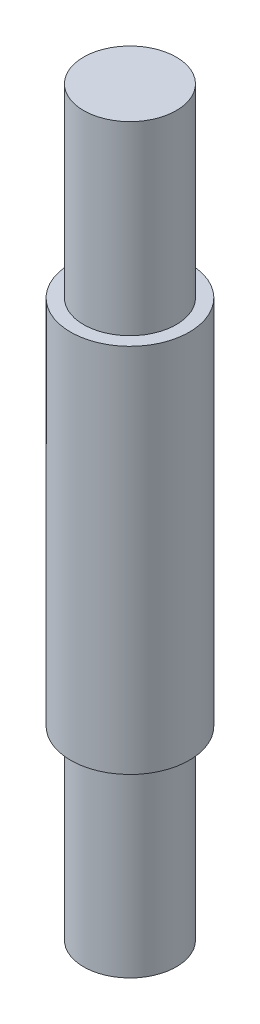
ISO-10303-21;
HEADER;
FILE_DESCRIPTION(('STEP AP214'),'2;1');
FILE_NAME('part.step','',(''),(''),'','','');
FILE_SCHEMA(('AUTOMOTIVE_DESIGN { 1 0 10303 214 1 1 1 1 }'));
ENDSEC;
DATA;
#1=APPLICATION_CONTEXT('core data for automotive mechanical design processes');
#2=APPLICATION_PROTOCOL_DEFINITION('international standard','automotive_design',2000,#1);
#3=PRODUCT_CONTEXT('',#1,'mechanical');
#4=PRODUCT('Part','Part','',(#3));
#5=PRODUCT_RELATED_PRODUCT_CATEGORY('part','',(#4));
#6=PRODUCT_DEFINITION_FORMATION('','',#4);
#7=PRODUCT_DEFINITION_CONTEXT('part definition',#1,'design');
#8=PRODUCT_DEFINITION('design','',#6,#7);
#9=PRODUCT_DEFINITION_SHAPE('','',#8);
#10=(LENGTH_UNIT() NAMED_UNIT(*) SI_UNIT(.MILLI.,.METRE.));
#11=(NAMED_UNIT(*) PLANE_ANGLE_UNIT() SI_UNIT($,.RADIAN.));
#12=(NAMED_UNIT(*) SI_UNIT($,.STERADIAN.) SOLID_ANGLE_UNIT());
#13=UNCERTAINTY_MEASURE_WITH_UNIT(LENGTH_MEASURE(1.E-05),#10,'distance_accuracy_value','');
#14=(GEOMETRIC_REPRESENTATION_CONTEXT(3) GLOBAL_UNCERTAINTY_ASSIGNED_CONTEXT((#13)) GLOBAL_UNIT_ASSIGNED_CONTEXT((#10,
#11,#12)) REPRESENTATION_CONTEXT('',''));
#15=CARTESIAN_POINT('',(0.,0.,0.));
#16=DIRECTION('',(0.,0.,1.));
#17=DIRECTION('',(1.,0.,0.));
#18=AXIS2_PLACEMENT_3D('',#15,#16,#17);
#19=CARTESIAN_POINT('',(0.,0.,0.));
#20=DIRECTION('',(0.,1.,0.));
#21=DIRECTION('',(-1.,0.,0.));
#22=AXIS2_PLACEMENT_3D('',#19,#20,#21);
#23=PLANE('',#22);
#24=CARTESIAN_POINT('',(0.,0.,0.));
#25=DIRECTION('',(0.,1.,0.));
#26=DIRECTION('',(-1.,0.,0.));
#27=AXIS2_PLACEMENT_3D('',#24,#25,#26);
#28=CIRCLE('',#27,12.5);
#29=CARTESIAN_POINT('',(-12.5,0.,0.));
#30=VERTEX_POINT('',#29);
#31=EDGE_CURVE('E10',#30,#30,#28,.T.);
#32=ORIENTED_EDGE('',*,*,#31,.F.);
#33=EDGE_LOOP('',(#32));
#34=FACE_BOUND('',#33,.T.);
#35=ADVANCED_FACE('F40',(#34),#23,.F.);
#36=CARTESIAN_POINT('',(0.,200.,0.));
#37=DIRECTION('',(0.,1.,0.));
#38=DIRECTION('',(-1.,0.,0.));
#39=AXIS2_PLACEMENT_3D('',#36,#37,#38);
#40=CYLINDRICAL_SURFACE('',#39,12.5);
#41=CARTESIAN_POINT('',(0.,50.,0.));
#42=DIRECTION('',(0.,1.,0.));
#43=DIRECTION('',(-1.,0.,0.));
#44=AXIS2_PLACEMENT_3D('',#41,#42,#43);
#45=CIRCLE('',#44,12.5);
#46=CARTESIAN_POINT('',(-12.5,50.,0.));
#47=VERTEX_POINT('',#46);
#48=EDGE_CURVE('E43',#47,#47,#45,.T.);
#49=ORIENTED_EDGE('',*,*,#48,.F.);
#50=EDGE_LOOP('',(#49));
#51=FACE_BOUND('',#50,.T.);
#52=ORIENTED_EDGE('',*,*,#31,.T.);
#53=EDGE_LOOP('',(#52));
#54=FACE_BOUND('',#53,.T.);
#55=ADVANCED_FACE('F83',(#51,#54),#40,.T.);
#56=CARTESIAN_POINT('',(12.5,50.,0.));
#57=DIRECTION('',(0.,1.,0.));
#58=DIRECTION('',(-1.,0.,0.));
#59=AXIS2_PLACEMENT_3D('',#56,#57,#58);
#60=PLANE('',#59);
#61=CARTESIAN_POINT('',(0.,50.,0.));
#62=DIRECTION('',(0.,1.,0.));
#63=DIRECTION('',(-1.,0.,0.));
#64=AXIS2_PLACEMENT_3D('',#61,#62,#63);
#65=CIRCLE('',#64,16.);
#66=CARTESIAN_POINT('',(-16.,50.,0.));
#67=VERTEX_POINT('',#66);
#68=EDGE_CURVE('E50',#67,#67,#65,.T.);
#69=ORIENTED_EDGE('',*,*,#68,.F.);
#70=EDGE_LOOP('',(#69));
#71=FACE_BOUND('',#70,.T.);
#72=ORIENTED_EDGE('',*,*,#48,.T.);
#73=EDGE_LOOP('',(#72));
#74=FACE_BOUND('',#73,.T.);
#75=ADVANCED_FACE('F78',(#71,#74),#60,.F.);
#76=CARTESIAN_POINT('',(0.,200.,0.));
#77=DIRECTION('',(0.,1.,0.));
#78=DIRECTION('',(-1.,0.,0.));
#79=AXIS2_PLACEMENT_3D('',#76,#77,#78);
#80=CYLINDRICAL_SURFACE('',#79,16.);
#81=CARTESIAN_POINT('',(0.,150.,0.));
#82=DIRECTION('',(0.,1.,0.));
#83=DIRECTION('',(-1.,0.,0.));
#84=AXIS2_PLACEMENT_3D('',#81,#82,#83);
#85=CIRCLE('',#84,16.);
#86=CARTESIAN_POINT('',(-16.,150.,0.));
#87=VERTEX_POINT('',#86);
#88=EDGE_CURVE('E51',#87,#87,#85,.T.);
#89=ORIENTED_EDGE('',*,*,#88,.F.);
#90=EDGE_LOOP('',(#89));
#91=FACE_BOUND('',#90,.T.);
#92=ORIENTED_EDGE('',*,*,#68,.T.);
#93=EDGE_LOOP('',(#92));
#94=FACE_BOUND('',#93,.T.);
#95=ADVANCED_FACE('F74',(#91,#94),#80,.T.);
#96=CARTESIAN_POINT('',(16.,150.,0.));
#97=DIRECTION('',(0.,-1.,0.));
#98=DIRECTION('',(1.,0.,0.));
#99=AXIS2_PLACEMENT_3D('',#96,#97,#98);
#100=PLANE('',#99);
#101=CARTESIAN_POINT('',(0.,150.,0.));
#102=DIRECTION('',(0.,1.,0.));
#103=DIRECTION('',(-1.,0.,0.));
#104=AXIS2_PLACEMENT_3D('',#101,#102,#103);
#105=CIRCLE('',#104,12.5);
#106=CARTESIAN_POINT('',(-12.5,150.,0.));
#107=VERTEX_POINT('',#106);
#108=EDGE_CURVE('E57',#107,#107,#105,.T.);
#109=ORIENTED_EDGE('',*,*,#108,.F.);
#110=EDGE_LOOP('',(#109));
#111=FACE_BOUND('',#110,.T.);
#112=ORIENTED_EDGE('',*,*,#88,.T.);
#113=EDGE_LOOP('',(#112));
#114=FACE_BOUND('',#113,.T.);
#115=ADVANCED_FACE('F69',(#111,#114),#100,.F.);
#116=CARTESIAN_POINT('',(0.,200.,0.));
#117=DIRECTION('',(0.,1.,0.));
#118=DIRECTION('',(-1.,0.,0.));
#119=AXIS2_PLACEMENT_3D('',#116,#117,#118);
#120=CYLINDRICAL_SURFACE('',#119,12.5);
#121=CARTESIAN_POINT('',(0.,200.,0.));
#122=DIRECTION('',(0.,1.,0.));
#123=DIRECTION('',(-1.,0.,0.));
#124=AXIS2_PLACEMENT_3D('',#121,#122,#123);
#125=CIRCLE('',#124,12.5);
#126=CARTESIAN_POINT('',(-12.5,200.,0.));
#127=VERTEX_POINT('',#126);
#128=EDGE_CURVE('E56',#127,#127,#125,.T.);
#129=ORIENTED_EDGE('',*,*,#128,.F.);
#130=EDGE_LOOP('',(#129));
#131=FACE_BOUND('',#130,.T.);
#132=ORIENTED_EDGE('',*,*,#108,.T.);
#133=EDGE_LOOP('',(#132));
#134=FACE_BOUND('',#133,.T.);
#135=ADVANCED_FACE('F63',(#131,#134),#120,.T.);
#136=CARTESIAN_POINT('',(12.5,200.,0.));
#137=DIRECTION('',(0.,-1.,0.));
#138=DIRECTION('',(1.,0.,0.));
#139=AXIS2_PLACEMENT_3D('',#136,#137,#138);
#140=PLANE('',#139);
#141=ORIENTED_EDGE('',*,*,#128,.T.);
#142=EDGE_LOOP('',(#141));
#143=FACE_BOUND('',#142,.T.);
#144=ADVANCED_FACE('F64',(#143),#140,.F.);
#145=CLOSED_SHELL('',(#35,#55,#75,#95,#115,#135,#144));
#146=MANIFOLD_SOLID_BREP('B2',#145);
#147=ADVANCED_BREP_SHAPE_REPRESENTATION('',(#18,#146),#14);
#148=SHAPE_DEFINITION_REPRESENTATION(#9,#147);
ENDSEC;
END-ISO-10303-21;
